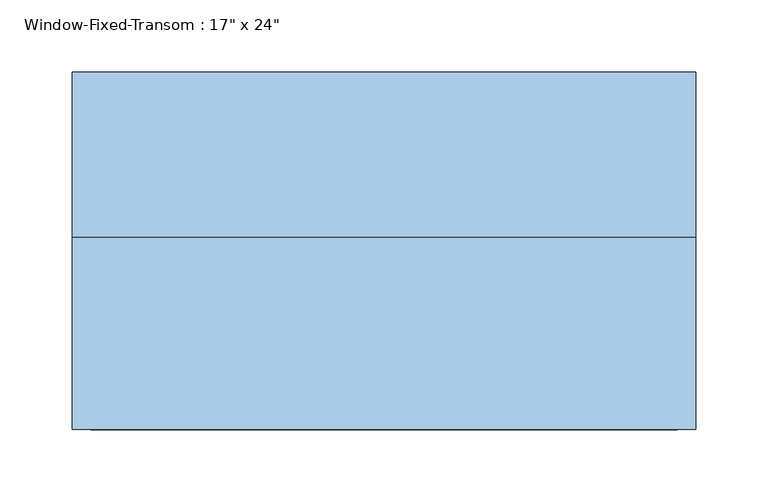
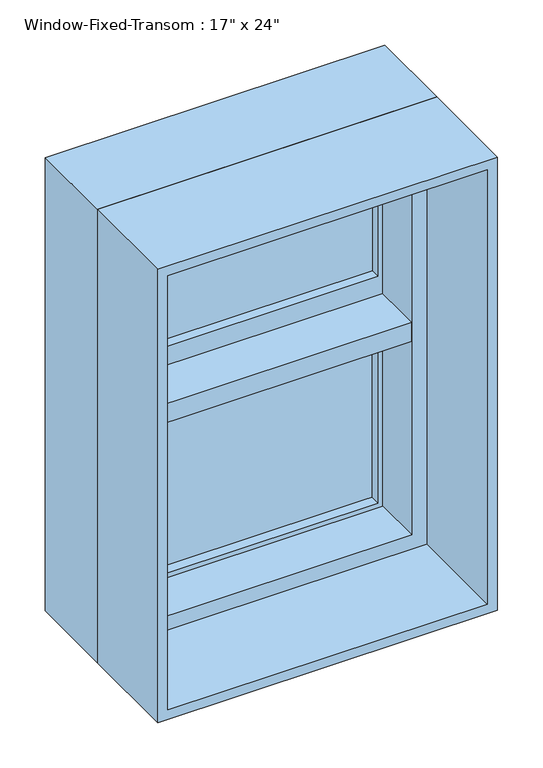
"""IFC4 building model written with IfcOpenShell, lengths in millimetres: window geometry."""

from ifc_helpers import new_model, si_unit, frame, origin, place, context, project, spatial, polyline, outline, extrude, faceted_brep, source, transform, mapped, element, save


def window_608ea798(model_context):
    return source(origin(), model_context, "Body", "SolidModel", [
        faceted_brep([(215.9, 19.05, 1524.0), (215.9, 133.35, 1524.0), (-215.9, 133.35, 1524.0), (-215.9, 19.05, 1524.0), (-215.9, 133.35, 914.4), (-215.9, 19.05, 914.4), (215.9, 133.35, 914.4), (215.9, 19.05, 914.4), (184.15, 19.05, 1492.25), (184.15, 19.05, 946.15), (-184.15, 19.05, 946.15), (-184.15, 19.05, 1492.25), (-203.2, 133.35, 1511.3), (-203.2, 133.35, 927.1), (203.2, 133.35, 927.1), (203.2, 133.35, 1511.3), (184.15, 82.55, 1492.25), (-184.15, 82.55, 1492.25), (203.2, 82.55, 1511.3), (-203.2, 82.55, 1511.3), (-184.15, 82.55, 946.15), (-203.2, 82.55, 927.1), (184.15, 82.55, 946.15), (203.2, 82.55, 927.1)], [[[0, 1, 2, 3]], [[3, 2, 4, 5]], [[5, 4, 6, 7]], [[3, 5, 7, 0], [8, 9, 10, 11]], [[7, 6, 1, 0]], [[1, 6, 4, 2], [12, 13, 14, 15]], [[16, 8, 11, 17]], [[15, 18, 19, 12]], [[17, 11, 10, 20]], [[12, 19, 21, 13]], [[20, 10, 9, 22]], [[13, 21, 23, 14]], [[22, 9, 8, 16]], [[18, 23, 21, 19], [17, 20, 22, 16]], [[14, 23, 18, 15]]]),
        extrude(outline(polyline([(1524.0, -215.9), (914.4, -215.9), (914.4, 215.9), (1524.0, 215.9), (1524.0, -215.9)]), holes=[polyline([(1511.3, 203.2), (927.1, 203.2), (927.1, -203.2), (1511.3, -203.2), (1511.3, 203.2)])]), frame((0.0, -114.3, 0.0), z_axis=(0.0, 1.0, 0.0), x_axis=(0.0, 0.0, 1.0)), (0.0, 0.0, 1.0), 133.35),
        extrude(outline(polyline([(927.1, 203.2), (1206.5, 203.2), (1206.5, -203.2), (927.1, -203.2), (927.1, 203.2)]), holes=[polyline([(952.5, -177.8), (1181.1, -177.8), (1181.1, 177.8), (952.5, 177.8), (952.5, -177.8)])]), frame((0.0, 82.55, 0.0), z_axis=(0.0, 1.0, 0.0), x_axis=(0.0, 0.0, 1.0)), (0.0, 0.0, 1.0), 44.45),
        extrude(outline(polyline([(177.8, 114.3), (177.8, 107.95), (-177.8, 107.95), (-177.8, 114.3), (177.8, 114.3)])), frame((0.0, 0.0, 952.5), z_axis=(0.0, 0.0, 1.0), x_axis=(1.0, 0.0, 0.0)), (0.0, 0.0, 1.0), 254.0),
        extrude(outline(polyline([(-177.8, 95.25), (-177.8, 101.6), (177.8, 101.6), (177.8, 95.25), (-177.8, 95.25)])), frame((0.0, 0.0, 952.5), z_axis=(0.0, 0.0, 1.0), x_axis=(1.0, 0.0, 0.0)), (0.0, 0.0, 1.0), 254.0),
        extrude(outline(polyline([(203.2, 127.0), (203.2, 82.55), (184.15, 82.55), (184.15, 19.05), (-184.15, 19.05), (-184.15, 82.55), (-203.2, 82.55), (-203.2, 127.0), (203.2, 127.0)])), frame((0.0, 0.0, 1206.5), z_axis=(0.0, 0.0, 1.0), x_axis=(1.0, 0.0, 0.0)), (0.0, 0.0, 1.0), 25.4),
        extrude(outline(polyline([(177.8, 114.3), (177.8, 107.95), (-177.8, 107.95), (-177.8, 114.3), (177.8, 114.3)])), frame((0.0, 0.0, 1257.3), z_axis=(0.0, 0.0, 1.0), x_axis=(1.0, 0.0, 0.0)), (0.0, 0.0, 1.0), 228.6),
        extrude(outline(polyline([(177.8, 101.6), (177.8, 95.25), (-177.8, 95.25), (-177.8, 101.6), (177.8, 101.6)])), frame((0.0, 0.0, 1257.3), z_axis=(0.0, 0.0, 1.0), x_axis=(1.0, 0.0, 0.0)), (0.0, 0.0, 1.0), 228.6),
        extrude(outline(polyline([(1511.3, -203.2), (1231.9, -203.2), (1231.9, 203.2), (1511.3, 203.2), (1511.3, -203.2)]), holes=[polyline([(1485.9, 177.8), (1257.3, 177.8), (1257.3, -177.8), (1485.9, -177.8), (1485.9, 177.8)])]), frame((0.0, 82.55, 0.0), z_axis=(0.0, 1.0, 0.0), x_axis=(0.0, 0.0, 1.0)), (0.0, 0.0, 1.0), 44.45),
    ])


if __name__ == "__main__":
    model = new_model("IFC4")
    model_context = context("Model", 3, world=origin())
    ifc_project = project(units=[si_unit("LENGTHUNIT", "METRE", prefix="MILLI")], contexts=[model_context])
    site = spatial("IfcSite", under=ifc_project)
    building = spatial("IfcBuilding", under=site)
    placement = place(None, origin())
    window_shape = window_608ea798(model_context)
    element("IfcWindow", 1, ObjectType="Window-Fixed-Transom : 17\" x 24\"", at=placement, inside=building, context=model_context, shape_type="MappedRepresentation", body=[
        mapped(window_shape, transform((0.0, 0.0, 0.0), x_axis=(1.0, 0.0, 0.0), y_axis=(0.0, 1.0, 0.0), z_axis=(0.0, 0.0, 1.0))),
    ])
    save(model, "model.ifc")

# Revit data of these elements
# Type "Window-Fixed-Transom : 17\" x 24\""
#   Type Mark = "19"
#   Fire Rating = "0.5h"
#   Assembly Code = "B2020100"
#   Analytic Construction = "Double glazing - domestic"
#   Window Inset [instance default] = 0' - 0"
#   Wall Thickness [instance default] = 0' - 6"
#   Visual Light Transmittance = 0.81
#   Transom Height = 1' - 0"
#   Thermal Resistance (R) = 1.8146 (h·ft²·°F)/BTU
#   Solar Heat Gain Coefficient = 0.76
#   Rough Width = 1' - 5 1/2"
#   Rough Height = 2' - 0 1/2"
#   Lower Sash Height = 1' - 0"
#   Interior Wall Closure [instance default] = 0' - 2 1/4"
#   Height = 2' - 0"
#   Heat Transfer Coefficient (U) = 0.5511 BTU/(h·ft²·°F)
#   Frame Extension [instance default] = 0' - 0 1/4"
#   Exterior Wall Closure [instance default] = 0' - 1 1/4"
#   Extension Jamb [instance default] = 0' - 2 1/4"
#   Default Sill Height = 3' - 0"
#   Width = 1' - 5"
#   Muntin Visibility = yes
#   Interior Trim Visibility [instance default] = yes
#   Exterior Trim Visibility [instance default] = yes
#   Extension Jamb Visibility [instance default] = yes
#   Muntin Pattern = Muntin Pattern_2x2 : Muntin Pattern_2x2
#   Interior Trim Material = Wood - Stained
#   Interior Trim = Trim-Window-Interior-Flat : Picture Frame
#   Interior Frame Material = Wood - Stained
#   Glass Panel Material = Glass
#   Exterior Trim Material = Clad - White
#   Exterior Trim = Trim-Window-Exterior-Flat : with Sill
#   Exterior Frame Material = Clad - White
#   Wall Closure = (empty or 0)
# Element 1 (IfcWindow, "Window-Fixed-Transom : 17\" x 24\"")
#   Wall Thickness = 0' - 9"
#   Extension Jamb = 0' - 5 1/4"
#   Materials on its faces: "Wood - Stained", "Glass", "Clad - White"
# Materials
#   "Wood - Stained": class "Wood", colour RGB 224 178 126, transparency 0, Cost = 0
#   "Glass": class "Glass", colour RGB 0 128 192, transparency 0.75, Description = "Soda Lime Glass", Cost = 0
#   "Clad - White": class "Wood", colour RGB 242 242 238, transparency 0, Cost = 0
